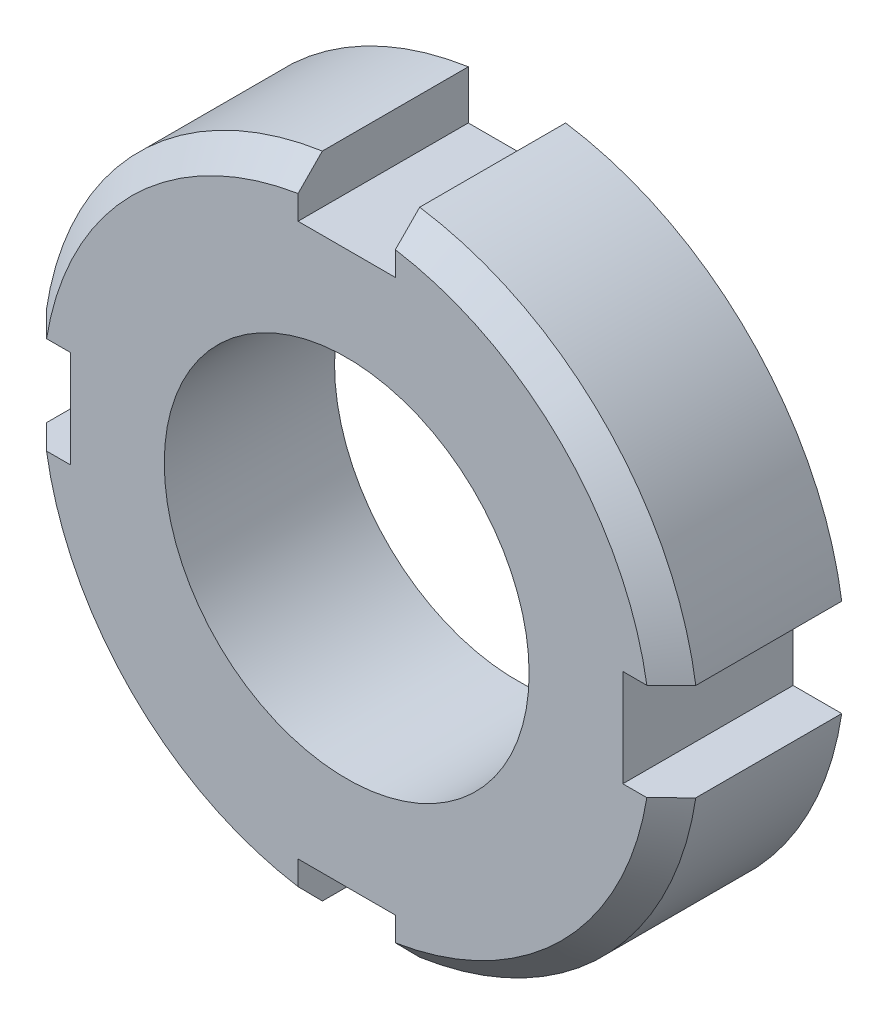
from build123d import *

# Parameters (mm, degrees)
NUT_BODY_7MM_DEPTH      = 3.5
BORE_15_DEPTH           = 21.137030566
BORE_15_DEPTH_BACK      = 21.137030566
BORE_SKETCH_15_R        = 7.5
EDGE_CHAMFERS_1X45_SIZE = 1


with BuildPart() as part:
    # Slotted Nut Profile Ø27 → Nut Body 7mm (new, symmetric)
    with BuildSketch(Plane.XY):
        with BuildLine():
            Line((2, 11.351029923), (2, 13.351029923))
            ThreePointArc((2, 13.351029923), (9.545941546, 9.545941546), (13.351029923, 2))
            Line((13.351029923, 2), (11.351029923, 2))
            Line((11.351029923, 2), (11.351029923, -2))
            Line((11.351029923, -2), (13.351029923, -2))
            ThreePointArc((13.351029923, -2), (9.545941546, -9.545941546), (2, -13.351029923))
            Line((2, -13.351029923), (2, -11.351029923))
            Line((2, -11.351029923), (-2, -11.351029923))
            Line((-2, -11.351029923), (-2, -13.351029923))
            ThreePointArc((-2, -13.351029923), (-9.545941546, -9.545941546), (-13.351029923, -2))
            Line((-13.351029923, -2), (-11.351029923, -2))
            Line((-11.351029923, -2), (-11.351029923, 2))
            Line((-11.351029923, 2), (-13.351029923, 2))
            ThreePointArc((-13.351029923, 2), (-9.545941546, 9.545941546), (-2, 13.351029923))
            Line((-2, 13.351029923), (-2, 11.351029923))
            Line((-2, 11.351029923), (2, 11.351029923))
        make_face()
    extrude(amount=NUT_BODY_7MM_DEPTH, both=True)

    # Bore Sketch Ø15 → Bore Ø15 (cut, two sides: drawn at the far end of the back side and taken through both)
    with BuildSketch(Plane.XY.offset(3.5).offset(-BORE_15_DEPTH_BACK)):
        Circle(BORE_SKETCH_15_R)
    extrude(amount=BORE_15_DEPTH + BORE_15_DEPTH_BACK, mode=Mode.SUBTRACT)

    # Edge Chamfers 1x45°
    edge_chamfers_1x45_edges = [part.edges().sort_by_distance(p)[0] for p in [
        (-9.545941546, 9.545941546, 3.5),
        (-9.545941546, -9.545941546, 3.5),
        (9.545941546, -9.545941546, 3.5),
        (9.545941546, 9.545941546, 3.5),
    ]]
    chamfer(edge_chamfers_1x45_edges, length=EDGE_CHAMFERS_1X45_SIZE)


solid = part.part
